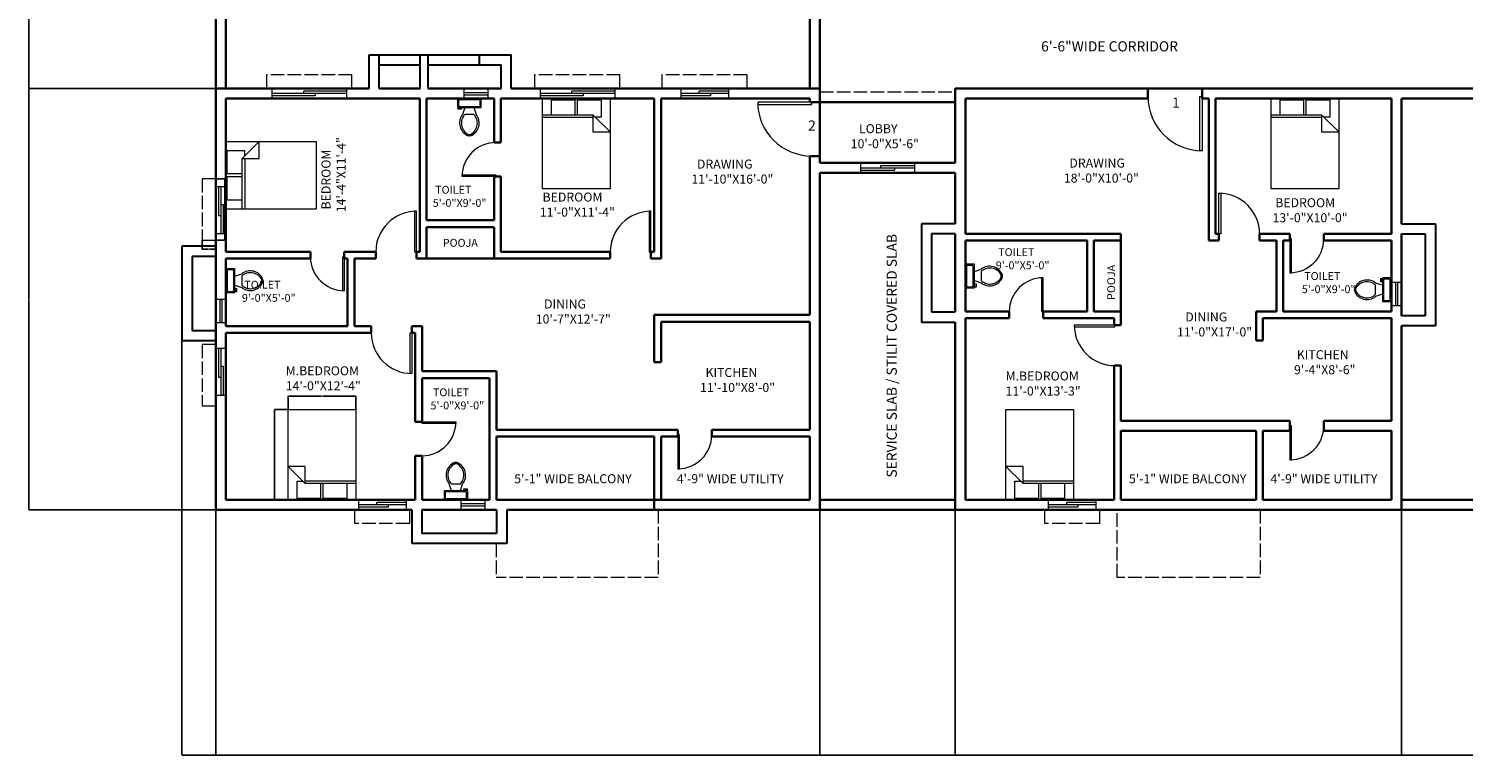
# Model space of a CAD drawing. Units: inches. Extents: x -69 to 2453, y 4803 to 7122.
# Tile 1 of 9: x -69 to 1203, y 4803 to 5448. Entities that reach past the tile are written whole.
import ezdxf

# ---------------------------------------------------------------- set-up
doc = ezdxf.new("R2010")
doc.units = ezdxf.units.IN
doc.linetypes.add('ACAD_ISO02W100', pattern=[15, 12, -3])
for name, color, linetype, lineweight in [('A-ANNO-DIMS', 2, 'Continuous', 18), ('A-ANNO-IDEN', 2, 'Continuous', 18), ('A-AREA-IDEN', 7, 'Continuous', 18), ('A-DOOR', 3, 'Continuous', 18), ('A-FLOR-FIXT', 9, 'Continuous', 18), ('A-FLOR-OVHD', 8, 'ACAD_ISO02W100', 13), ('A-FURN', 8, 'Continuous', 18), ('A-GLAZ', 244, 'Continuous', 18), ('A-WALL', 7, 'Continuous', 35), ('A-WALL-SRVC', 7, 'Continuous', 30)]:
    doc.layers.add(name, color=color, linetype=linetype, lineweight=lineweight)
doc.styles.get("Standard").update_dxf_attribs({"font": 'arial.ttf'})
doc.dimstyles.get("Standard").update_dxf_attribs({"dimtxt": 0.18, "dimasz": 0.18, "dimexe": 0.18, "dimexo": 0.0625, "dimgap": 0.09, "dimtad": 0, "dimtih": 1, "dimtoh": 1, "dimdec": 4, "dimzin": 0, "dimdsep": 46, "dimtxsty": 'Standard', "dimcen": 0.09, "dimadec": 0, "dimazin": 0, "dimtfac": 1, "dimtdec": 4, "dimtofl": 0, "dimtmove": 0, "dimatfit": 3, "dimfxl": 1, "dimtolj": 1, "dimtzin": 0, "dimarcsym": 0})

# ---------------------------------------------------------------- blocks, each defined once
blk = doc.blocks.new('*U2')
for p, q in [((-40, 0), (-40, 6)), ((0, 0), (0, 6))]:
    blk.add_line(p, q)
blk.add_lwpolyline([(0, 0), (0, -40), (-1.75, -40), (-1.75, 0)], close=True)
blk.add_arc((0, 0), 40, 180, 270)
blk = doc.blocks.new('*U4')
for p, q in [((0, 0), (0, -6)), ((-40, 0), (-40, -6))]:
    blk.add_line(p, q)
blk.add_lwpolyline([(0, 0), (0, 40), (-1.75, 40), (-1.75, 0)], close=True)
blk.add_arc((0, 0), 40, 90, 180)
blk = doc.blocks.new('*U3')
for p, q in [((0, 0), (0, 6)), ((40, 0), (40, 6))]:
    blk.add_line(p, q)
blk.add_lwpolyline([(0, 0), (0, -40), (1.75, -40), (1.75, 0)], close=True)
blk.add_arc((0, 0), 40, 270, 360)
blk = doc.blocks.new('*U6')
for p, q in [((-40, 0), (-40, 6)), ((0, 0), (0, 6))]:
    blk.add_line(p, q)
blk.add_lwpolyline([(0, 0), (0, -40), (-1.75, -40), (-1.75, 0)], close=True)
blk.add_arc((0, 0), 40, 180, 270)
blk = doc.blocks.new('*U17')
for p, q in [((0, 0), (0, 6)), ((40, 0), (40, 6))]:
    blk.add_line(p, q)
blk.add_lwpolyline([(0, 0), (0, -40), (1.75, -40), (1.75, 0)], close=True)
blk.add_arc((0, 0), 40, 270, 0)
blk = doc.blocks.new('*U5')
for p, q in [((0, 0), (0, -6)), ((40, 0), (40, -6))]:
    blk.add_line(p, q)
blk.add_lwpolyline([(0, 0), (0, 40), (1.75, 40), (1.75, 0)], close=True)
blk.add_arc((0, 0), 40, 0, 90)
blk = doc.blocks.new('*U21')
for p, q in [((-40, 0), (-40, -6)), ((0, 0), (0, -6))]:
    blk.add_line(p, q)
blk.add_lwpolyline([(0, 0), (0, 40), (-1.75, 40), (-1.75, 0)], close=True)
blk.add_arc((0, 0), 40, 90, 180)
blk = doc.blocks.new('Bed - Queen')
for p, q in [((0, -80.00003), (0, 0)), ((0, 0), (59.99999, 0)), ((59.99999, 0), (59.99999, -80.00003)), ((7.99999, -1.2), (28.79998, -1.2)), ((7.99999, -14.4), (7.99999, -1.2)), ((28.79998, -1.2), (28.79998, -14.4)), ((31.19999, -1.2), (51.99999, -1.2)), ((31.19999, -14.4), (31.19999, -1.2)), ((51.99999, -1.2), (51.99999, -16.4)), ((0, -14.4), (44.8, -14.4)), ((44.8, -16.8), (0, -16.8)), ((59.99999, -29.6), (44.8, -14.4)), ((44.8, -14.4), (44.8, -29.6)), ((51.99999, -16.4), (46.79936, -16.4)), ((44.8, -29.6), (59.99999, -29.6)), ((59.99999, -80.00003), (0, -80.00003))]:
    blk.add_line(p, q)
blk = doc.blocks.new('*U33')
for p, q in [((-10, -8.5), (-8, -8.5)), ((-10, -9.5), (-10, -8.5)), ((-7, -9.5), (-10, -9.5)), ((-8, -8.5), (-8, -8)), ((-7, -8), (-7, -9.5)), ((-4, -8), (-6, -14)), ((4, -8), (6, -14)), ((9.5, -6), (9.5, -2)), ((4, -14), (-4, -14))]:
    blk.add_line(p, q)
blk.add_lwpolyline([(10.5, -8), (10.5, 0), (-10.5, 0), (-10.5, -8)], close=True)
for points in [[(-9.5, -2), (-9.5, -6)], [(8.5, -1), (-8.5, -1)], [(-8.5, -7), (8.5, -7)]]:
    blk.add_lwpolyline(points)
for centre, radius, start, end in [((-8.6, -1.9), 0.884, 81.8699, 188.1301), ((-8.6, -6.1), 0.884, 171.8699, 278.1301), ((8.6, -1.9), 0.884, 351.8699, 98.1301), ((8.6, -6.1), 0.884, 261.8699, 8.1301), ((3.5, -21.6), 12.2, 141.4691, 247.9714), ((4.2, -21.8), 11.3, 136.3677, 238.9468), ((-3.5, -21.6), 12.2, 292.0284, 38.5307), ((-4.2, -21.8), 11.3, 301.053, 43.6321), ((0, -27.9), 4, 245.7318, 294.2682), ((0, -29), 4, 254.8605, 285.1395)]:
    blk.add_arc(centre, radius, start, end)
blk = doc.blocks.new('WINDOW-VENT-21IN')
for p, q in [((0, 5.5), (21, 5.5)), ((0, 3.5), (21, 3.5))]:
    blk.add_line(p, q)
blk.add_lwpolyline([(0, 9), (21, 9), (21, 0), (0, 0)], close=True)
blk = doc.blocks.new('WINDOW-SLIDING-42IN')
for p, q in [((2.5, 42), (2.5, 16)), ((4.5, 42), (4.5, 0)), ((4.5, 26), (6.5, 26)), ((6.5, 26), (6.5, 0)), ((4.5, 16), (2.5, 16))]:
    blk.add_line(p, q)
blk.add_lwpolyline([(0, 42), (9, 42), (9, 0), (0, 0)], close=True)
blk = doc.blocks.new('WINDOW-SLIDING-66IN')
for p, q in [((66, 4.5), (0, 4.5)), ((38, 2.5), (0, 2.5)), ((66, 6.5), (28, 6.5)), ((28, 4.5), (28, 6.5)), ((38, 4.5), (38, 2.5))]:
    blk.add_line(p, q)
blk.add_lwpolyline([(66, 9), (66, 0), (0, 0), (0, 9)], close=True)
blk = doc.blocks.new('SUNSHADE-54IN')
for p, q in [((12, 54.3), (0, 54.3)), ((0, 54.3), (0, 0)), ((0, 0), (12, 0))]:
    blk.add_line(p, q)
blk = doc.blocks.new('SUNSHADE-48IN')
for p, q in [((0, 0), (0, 12)), ((48.4, 0), (0, 0)), ((48.4, 12), (48.4, 0))]:
    blk.add_line(p, q)
blk = doc.blocks.new('SUNSHADE-76IN')
for p, q in [((75.7, 12), (0, 12)), ((0, 12), (0, 0)), ((75.7, 0), (75.7, 12))]:
    blk.add_line(p, q)
blk = doc.blocks.new('SERVICE-BAY-87IN')
for p, q in [((30, 87.2), (0, 87.2)), ((0, 87.2), (0, 0)), ((30, 78.2), (9, 78.2)), ((9, 78.2), (9, 9)), ((0, 0), (30, 0)), ((9, 9), (30, 9))]:
    blk.add_line(p, q)
blk = doc.blocks.new('*D51')
at = {"layer": 'A-ANNO-DIMS', "color": 0, "lineweight": -2, "transparency": 16777216}
for p, q in [((160.6, 5109.7), (148.5, 5109.7)), ((148.7, 5109.5), (148.7, 5069.9)), ((148.7, 5029.9), (148.7, 5069.5)), ((160.6, 5029.7), (148.5, 5029.7))]:
    blk.add_line(p, q, dxfattribs=at)
at = {"layer": 'A-ANNO-DIMS', "color": 0, "transparency": 16777216}
for points in [[(148.7, 5109.5), (148.7, 5109.5), (148.7, 5109.7)], [(148.7, 5029.9), (148.7, 5029.9), (148.7, 5029.7)]]:
    blk.add_solid(points, dxfattribs=at)
at = {"layer": 'Defpoints', "color": 0, "transparency": 16777216}
for p in [(160.7, 5109.7), (148.7, 5029.7), (160.7, 5029.7)]:
    blk.add_point(p, dxfattribs=at)
at = {"layer": 'A-ANNO-DIMS', "color": 0, "transparency": 16777216, "insert": (148.7, 5069.7), "char_height": 0.18, "attachment_point": 5}
blk.add_mtext('\\A1;QUEEN BED 80 TYP.', dxfattribs=at)
blk = doc.blocks.new('*D52')
at = {"layer": 'A-ANNO-DIMS', "color": 0, "lineweight": -2, "transparency": 16777216}
for p, q in [((160.7, 5109.8), (160.7, 5121.9)), ((160.9, 5121.7), (190.2, 5121.7)), ((220.5, 5121.7), (191.2, 5121.7)), ((220.7, 5109.8), (220.7, 5121.9))]:
    blk.add_line(p, q, dxfattribs=at)
at = {"layer": 'A-ANNO-DIMS', "color": 0, "transparency": 16777216}
for points in [[(160.9, 5121.7), (160.9, 5121.7), (160.7, 5121.7)], [(220.5, 5121.7), (220.5, 5121.7), (220.7, 5121.7)]]:
    blk.add_solid(points, dxfattribs=at)
at = {"layer": 'Defpoints', "color": 0, "transparency": 16777216}
for p in [(160.7, 5121.7), (160.7, 5109.7), (220.7, 5109.7)]:
    blk.add_point(p, dxfattribs=at)
at = {"layer": 'A-ANNO-DIMS', "color": 0, "transparency": 16777216, "insert": (190.7, 5121.7), "char_height": 0.18, "attachment_point": 5}
blk.add_mtext('\\A1;60 TYP.', dxfattribs=at)
blk = doc.blocks.new('*D59')
at = {"layer": 'A-ANNO-DIMS', "color": 0, "lineweight": -2, "transparency": 16777216}
for p, q in [((96.6, 5314.5), (104.8, 5314.5)), ((104.7, 5314.3), (104.7, 5287.5)), ((104.7, 5260.4), (104.7, 5287.2)), ((96.6, 5260.2), (104.8, 5260.2))]:
    blk.add_line(p, q, dxfattribs=at)
at = {"layer": 'A-ANNO-DIMS', "color": 0, "transparency": 16777216}
for points in [[(104.6, 5314.3), (104.7, 5314.3), (104.7, 5314.5)], [(104.6, 5260.4), (104.7, 5260.4), (104.7, 5260.2)]]:
    blk.add_solid(points, dxfattribs=at)
at = {"layer": 'Defpoints', "color": 0, "transparency": 16777216}
for p in [(96.5, 5314.5), (104.7, 5314.5), (96.5, 5260.2)]:
    blk.add_point(p, dxfattribs=at)
at = {"layer": 'A-ANNO-DIMS', "color": 0, "transparency": 16777216, "insert": (104.7, 5287.4), "char_height": 0.18, "attachment_point": 5}
blk.add_mtext('\\A1;SUNSHADE 54 TYP.', dxfattribs=at)
blk = doc.blocks.new('*D60')
at = {"layer": 'A-ANNO-DIMS', "color": 0, "lineweight": -2, "transparency": 16777216}
for p, q in [((84.5, 5260.1), (84.5, 5251.9)), ((96.5, 5260.1), (96.5, 5251.9)), ((84.7, 5252), (90, 5252)), ((96.3, 5252), (91, 5252))]:
    blk.add_line(p, q, dxfattribs=at)
at = {"layer": 'A-ANNO-DIMS', "color": 0, "transparency": 16777216}
for points in [[(84.7, 5252.1), (84.7, 5252), (84.5, 5252)], [(96.3, 5252.1), (96.3, 5252), (96.5, 5252)]]:
    blk.add_solid(points, dxfattribs=at)
at = {"layer": 'Defpoints', "color": 0, "transparency": 16777216}
for p in [(84.5, 5260.2), (96.5, 5260.2), (96.5, 5252)]:
    blk.add_point(p, dxfattribs=at)
at = {"layer": 'A-ANNO-DIMS', "color": 0, "transparency": 16777216, "insert": (90.5, 5252), "char_height": 0.18, "attachment_point": 5}
blk.add_mtext('\\A1;12 TYP.', dxfattribs=at)
blk = doc.blocks.new('*D81')
at = {"layer": 'A-ANNO-DIMS', "color": 0, "lineweight": -2, "transparency": 16777216}
for p, q in [((96.5, 5020.7), (96.5, 4802.8)), ((632.5, 5020.7), (632.5, 4802.8)), ((96.7, 4803), (364.2, 4803)), ((632.3, 4803), (364.8, 4803))]:
    blk.add_line(p, q, dxfattribs=at)
at = {"layer": 'A-ANNO-DIMS', "color": 0, "transparency": 16777216}
for points in [[(96.7, 4803), (96.7, 4802.9), (96.5, 4803)], [(632.3, 4803), (632.3, 4802.9), (632.5, 4803)]]:
    blk.add_solid(points, dxfattribs=at)
at = {"layer": 'Defpoints', "color": 0, "transparency": 16777216}
for p in [(96.5, 5020.7), (632.5, 5020.7), (632.5, 4803)]:
    blk.add_point(p, dxfattribs=at)
at = {"layer": 'A-ANNO-DIMS', "color": 0, "transparency": 16777216, "insert": (364.5, 4803), "char_height": 0.18, "attachment_point": 5}
blk.add_mtext('\\A1;536', dxfattribs=at)
blk = doc.blocks.new('*D82')
at = {"layer": 'A-ANNO-DIMS', "color": 0, "lineweight": -2, "transparency": 16777216}
for p, q in [((632.5, 5020.7), (632.5, 4802.8)), ((752.5, 5020.7), (752.5, 4802.8)), ((632.7, 4803), (692.2, 4803)), ((752.3, 4803), (692.8, 4803))]:
    blk.add_line(p, q, dxfattribs=at)
at = {"layer": 'A-ANNO-DIMS', "color": 0, "transparency": 16777216}
for points in [[(632.7, 4803), (632.7, 4802.9), (632.5, 4803)], [(752.3, 4803), (752.3, 4802.9), (752.5, 4803)]]:
    blk.add_solid(points, dxfattribs=at)
at = {"layer": 'Defpoints', "color": 0, "transparency": 16777216}
for p in [(632.5, 5020.7), (752.5, 5020.7), (752.5, 4803)]:
    blk.add_point(p, dxfattribs=at)
at = {"layer": 'A-ANNO-DIMS', "color": 0, "transparency": 16777216, "insert": (692.5, 4803), "char_height": 0.18, "attachment_point": 5}
blk.add_mtext('\\A1;120', dxfattribs=at)
blk = doc.blocks.new('*D83')
at = {"layer": 'A-ANNO-DIMS', "color": 0, "lineweight": -2, "transparency": 16777216}
for p, q in [((752.5, 5020.7), (752.5, 4802.8)), ((1148.5, 5020.7), (1148.5, 4802.8)), ((752.7, 4803), (950.2, 4803)), ((1148.3, 4803), (950.8, 4803))]:
    blk.add_line(p, q, dxfattribs=at)
at = {"layer": 'A-ANNO-DIMS', "color": 0, "transparency": 16777216}
for points in [[(752.7, 4803), (752.7, 4802.9), (752.5, 4803)], [(1148.3, 4803), (1148.3, 4802.9), (1148.5, 4803)]]:
    blk.add_solid(points, dxfattribs=at)
at = {"layer": 'Defpoints', "color": 0, "transparency": 16777216}
for p in [(752.5, 5020.7), (1148.5, 5020.7), (1148.5, 4803)]:
    blk.add_point(p, dxfattribs=at)
at = {"layer": 'A-ANNO-DIMS', "color": 0, "transparency": 16777216, "insert": (950.5, 4803), "char_height": 0.18, "attachment_point": 5}
blk.add_mtext('\\A1;396', dxfattribs=at)
blk = doc.blocks.new('*D84')
at = {"layer": 'A-ANNO-DIMS', "color": 0, "lineweight": -2, "transparency": 16777216}
for p, q in [((1148.5, 5020.7), (1148.5, 4802.8)), ((1277.5, 5020.7), (1277.5, 4802.8)), ((1148.7, 4803), (1212.7, 4803)), ((1277.3, 4803), (1213.3, 4803))]:
    blk.add_line(p, q, dxfattribs=at)
at = {"layer": 'A-ANNO-DIMS', "color": 0, "transparency": 16777216}
for points in [[(1148.7, 4803), (1148.7, 4802.9), (1148.5, 4803)], [(1277.3, 4803), (1277.3, 4802.9), (1277.5, 4803)]]:
    blk.add_solid(points, dxfattribs=at)
at = {"layer": 'Defpoints', "color": 0, "transparency": 16777216}
for p in [(1148.5, 5020.7), (1277.5, 5020.7), (1277.5, 4803)]:
    blk.add_point(p, dxfattribs=at)
at = {"layer": 'A-ANNO-DIMS', "color": 0, "transparency": 16777216, "insert": (1213, 4803), "char_height": 0.18, "attachment_point": 5}
blk.add_mtext('\\A1;129', dxfattribs=at)
blk = doc.blocks.new('*D95')
at = {"layer": 'A-ANNO-DIMS', "color": 0, "lineweight": -2, "transparency": 16777216}
for p, q in [((96.509262, 5020.652777), (96.509262, 4802.785277)), ((2286.509262, 4977.652777), (2286.509262, 4802.785277)), ((96.689262, 4802.965277), (1191.149262, 4802.965277)), ((2286.329262, 4802.965277), (1191.869262, 4802.965277))]:
    blk.add_line(p, q, dxfattribs=at)
at = {"layer": 'A-ANNO-DIMS', "color": 0, "transparency": 16777216}
for points in [[(96.689262, 4802.995277), (96.689262, 4802.935277), (96.509262, 4802.965277)], [(2286.329262, 4802.995277), (2286.329262, 4802.935277), (2286.509262, 4802.965277)]]:
    blk.add_solid(points, dxfattribs=at)
at = {"layer": 'Defpoints', "color": 0, "transparency": 16777216}
for p in [(96.509262, 5020.715277), (2286.509262, 4977.715277), (2286.509262, 4802.965277)]:
    blk.add_point(p, dxfattribs=at)
at = {"layer": 'A-ANNO-DIMS', "color": 0, "transparency": 16777216, "insert": (1191.509262, 4802.965277), "char_height": 0.18, "attachment_point": 5}
blk.add_mtext('\\A1;2190', dxfattribs=at)
blk = doc.blocks.new('*D97')
at = {"layer": 'A-ANNO-DIMS', "color": 0, "lineweight": -2, "transparency": 16777216}
for p, q in [((96.4, 5394.7), (-69.4, 5394.7)), ((-69.2, 5394.5), (-69.2, 5207.9)), ((-69.2, 5020.9), (-69.2, 5207.5)), ((96.4, 5020.7), (-69.4, 5020.7))]:
    blk.add_line(p, q, dxfattribs=at)
at = {"layer": 'A-ANNO-DIMS', "color": 0, "transparency": 16777216}
for points in [[(-69.3, 5394.5), (-69.2, 5394.5), (-69.2, 5394.7)], [(-69.3, 5020.9), (-69.2, 5020.9), (-69.2, 5020.7)]]:
    blk.add_solid(points, dxfattribs=at)
at = {"layer": 'Defpoints', "color": 0, "transparency": 16777216}
for p in [(-69.2, 5394.7), (96.5, 5394.7), (96.5, 5020.7)]:
    blk.add_point(p, dxfattribs=at)
at = {"layer": 'A-ANNO-DIMS', "color": 0, "transparency": 16777216, "insert": (-69.2, 5207.7), "char_height": 0.18, "attachment_point": 5}
blk.add_mtext('\\A1;374', dxfattribs=at)
blk = doc.blocks.new('*D98')
at = {"layer": 'A-ANNO-DIMS', "color": 0, "lineweight": -2, "transparency": 16777216}
for p, q in [((96.4, 5514.7), (-69.4, 5514.7)), ((-69.2, 5514.5), (-69.2, 5454.9)), ((-69.2, 5394.9), (-69.2, 5454.5)), ((96.4, 5394.7), (-69.4, 5394.7))]:
    blk.add_line(p, q, dxfattribs=at)
at = {"layer": 'A-ANNO-DIMS', "color": 0, "transparency": 16777216}
for points in [[(-69.3, 5514.5), (-69.2, 5514.5), (-69.2, 5514.7)], [(-69.3, 5394.9), (-69.2, 5394.9), (-69.2, 5394.7)]]:
    blk.add_solid(points, dxfattribs=at)
at = {"layer": 'Defpoints', "color": 0, "transparency": 16777216}
for p in [(-69.2, 5514.7), (96.5, 5514.7), (96.5, 5394.7)]:
    blk.add_point(p, dxfattribs=at)
at = {"layer": 'A-ANNO-DIMS', "color": 0, "transparency": 16777216, "insert": (-69.2, 5454.7), "char_height": 0.18, "attachment_point": 5}
blk.add_mtext('\\A1;120', dxfattribs=at)
blk = doc.blocks.new('*D105')
at = {"layer": 'A-ANNO-DIMS', "color": 0, "lineweight": -2, "transparency": 16777216}
for p, q in [((66.509262, 5170.610035), (66.509262, 4802.785277)), ((2316.509262, 5140.587945), (2316.509262, 4802.785277)), ((66.689262, 4802.965277), (1191.149262, 4802.965277)), ((2316.329262, 4802.965277), (1191.869262, 4802.965277))]:
    blk.add_line(p, q, dxfattribs=at)
at = {"layer": 'A-ANNO-DIMS', "color": 0, "transparency": 16777216}
for points in [[(66.689262, 4802.995277), (66.689262, 4802.935277), (66.509262, 4802.965277)], [(2316.329262, 4802.995277), (2316.329262, 4802.935277), (2316.509262, 4802.965277)]]:
    blk.add_solid(points, dxfattribs=at)
at = {"layer": 'Defpoints', "color": 0, "transparency": 16777216}
for p in [(66.509262, 5170.672535), (2316.509262, 5140.650445), (2316.509262, 4802.965277)]:
    blk.add_point(p, dxfattribs=at)
at = {"layer": 'A-ANNO-DIMS', "color": 0, "transparency": 16777216, "insert": (1191.509262, 4802.965277), "char_height": 0.18, "attachment_point": 5}
blk.add_mtext('\\A1;2250', dxfattribs=at)

msp = doc.modelspace()

# ---------------------------------------------------------------- linework, layer by layer
at = {"layer": 'A-FLOR-OVHD'}
for p, q in [((632.5, 5391.7), (752.5, 5391.7)), ((489, 5020.7), (489, 4960.7)), ((896.1, 4960.7), (896.1, 5020.7)), ((1023, 5020.7), (1023, 4960.7)), ((345.4, 4990.7), (345.4, 4960.7)), ((489, 4960.7), (345.4, 4960.7)), ((1023, 4960.7), (896.1, 4960.7))]:
    msp.add_line(p, q, dxfattribs=at)
at = {"layer": 'A-GLAZ'}
for p, q in [((668.5, 5328.7), (668.5, 5319.7)), ((668.5, 5324.2), (716.5, 5324.2)), ((668.5, 5322.2), (698.5, 5322.2)), ((686.5, 5326.2), (716.5, 5326.2)), ((686.5, 5324.2), (686.5, 5326.2)), ((698.5, 5324.2), (698.5, 5322.2)), ((716.5, 5328.7), (716.5, 5319.7))]:
    msp.add_line(p, q, dxfattribs=at)
at = {"layer": 'A-WALL'}
for p, q in [((632.5, 6021.7), (632.5, 5328.7)), ((96.5, 5659.3), (96.5, 5020.7)), ((105.5, 5514.7), (105.5, 5394.7)), ((623.5, 5514.7), (623.5, 5394.7)), ((96.5, 5394.7), (232.6, 5394.7)), ((105.5, 5385.7), (277.5, 5385.7)), ((105.5, 5385.7), (105.5, 5249.7)), ((241.6, 5394.7), (277.8, 5394.7)), ((277.5, 5385.7), (277.5, 5249.7)), ((283.5, 5385.7), (283.5, 5277.7)), ((283.5, 5385.7), (343.5, 5385.7)), ((284.9, 5394.7), (349.7, 5394.7)), ((343.5, 5385.7), (343.5, 5346.7)), ((349.5, 5385.7), (349.5, 5346.7)), ((349.5, 5385.7), (485.5, 5385.7)), ((358.7, 5394.7), (632.5, 5394.7)), ((485.5, 5385.7), (485.5, 5249.7)), ((491.5, 5385.7), (623.5, 5385.7)), ((491.5, 5385.7), (491.5, 5243.7)), ((623.5, 5385.7), (623.5, 5382.7)), ((752.5, 5394.7), (752.5, 5328.7)), ((752.5, 5394.7), (1673.5, 5394.7)), ((761.5, 5385.7), (761.5, 5265.7)), ((761.5, 5385.7), (923.5, 5385.7)), ((923.5, 5385.7), (923.5, 5394.7)), ((971.5, 5385.7), (971.5, 5394.7)), ((971.5, 5385.7), (977.5, 5385.7)), ((977.5, 5385.7), (977.5, 5259.7)), ((983.5, 5385.7), (983.5, 5265.7)), ((983.5, 5385.7), (1139.5, 5385.7)), ((1139.5, 5385.7), (1139.5, 5265.7)), ((1148.5, 5385.7), (1277.5, 5385.7)), ((1148.5, 5385.7), (1148.5, 5274.7)), ((623.5, 5382.7), (752.5, 5382.7)), ((343.5, 5346.7), (349.5, 5346.7)), ((623.5, 5334.7), (632.5, 5334.7)), ((623.5, 5334.7), (623.5, 5193.7)), ((632.5, 5328.7), (752.5, 5328.7)), ((343.5, 5316.7), (349.5, 5316.7)), ((343.5, 5316.7), (343.5, 5277.7)), ((349.5, 5316.7), (349.5, 5249.7)), ((632.5, 5319.7), (752.5, 5319.7)), ((632.5, 5319.7), (632.5, 5020.7)), ((752.5, 5319.7), (752.5, 5274.6)), ((283.5, 5277.7), (343.5, 5277.7)), ((283.5, 5271.7), (343.5, 5271.7)), ((283.5, 5271.7), (283.5, 5243.7)), ((343.5, 5271.7), (343.5, 5243.7)), ((752.5, 5265.6), (752.5, 5196.4)), ((761.5, 5265.7), (899.5, 5265.7)), ((761.5, 5259.7), (869.5, 5259.7)), ((761.5, 5259.7), (761.5, 5196.7)), ((869.5, 5259.7), (869.5, 5196.7)), ((875.5, 5259.7), (875.5, 5196.7)), ((875.5, 5259.7), (899.5, 5259.7)), ((899.5, 5265.7), (899.5, 5184.7)), ((977.5, 5259.7), (986.5, 5259.7)), ((983.5, 5265.7), (986.5, 5265.7)), ((986.5, 5265.7), (986.5, 5259.7)), ((1022.5, 5265.7), (1022.5, 5259.7)), ((1022.5, 5265.7), (1049.5, 5265.7)), ((1022.5, 5259.7), (1037.5, 5259.7)), ((1037.5, 5259.7), (1037.5, 5196.7)), ((1043.5, 5259.7), (1043.5, 5196.7)), ((1043.5, 5259.7), (1049.5, 5259.7)), ((1049.5, 5259.7), (1049.5, 5265.7)), ((1079.5, 5259.7), (1079.5, 5265.7)), ((1079.5, 5265.7), (1139.5, 5265.7)), ((1079.5, 5259.7), (1139.5, 5259.7)), ((1139.5, 5259.7), (1139.5, 5196.7)), ((1148.5, 5265.7), (1148.5, 5193)), ((105.5, 5249.7), (180.5, 5249.7)), ((105.5, 5243.7), (180.5, 5243.7)), ((105.5, 5243.7), (105.5, 5183.7)), ((180.5, 5243.7), (180.5, 5249.7)), ((210.5, 5243.7), (210.5, 5249.7)), ((210.5, 5249.7), (238.5, 5249.7)), ((210.5, 5243.7), (213.5, 5243.7)), ((213.5, 5243.7), (213.5, 5183.7)), ((219.5, 5243.7), (219.5, 5183.7)), ((219.5, 5243.7), (238.5, 5243.7)), ((238.5, 5249.7), (238.5, 5243.7)), ((274.5, 5249.7), (274.5, 5243.7)), ((274.5, 5249.7), (277.5, 5249.7)), ((274.5, 5243.7), (446.5, 5243.7)), ((349.5, 5249.7), (446.5, 5249.7)), ((446.5, 5249.7), (446.5, 5243.7)), ((482.5, 5249.7), (482.5, 5243.7)), ((482.5, 5249.7), (485.5, 5249.7)), ((482.5, 5243.7), (491.5, 5243.7)), ((485.5, 5193.7), (623.5, 5193.7)), ((485.5, 5193.7), (485.5, 5151.7)), ((761.5, 5196.7), (800.5, 5196.7)), ((800.5, 5196.7), (800.5, 5190.7)), ((830.5, 5196.7), (830.5, 5190.7)), ((830.5, 5196.7), (869.5, 5196.7)), ((875.5, 5196.7), (899.5, 5196.7)), ((1019.5, 5196.7), (1037.5, 5196.7)), ((1019.5, 5196.7), (1019.5, 5170.9)), ((1043.5, 5196.7), (1139.5, 5196.7)), ((105.5, 5183.7), (213.5, 5183.7)), ((219.5, 5183.7), (234.5, 5183.7)), ((234.5, 5177.7), (234.5, 5183.7)), ((270.5, 5177.7), (270.5, 5183.7)), ((270.5, 5183.7), (279.5, 5183.7)), ((279.5, 5183.7), (279.5, 5143.7)), ((491.5, 5187.7), (623.5, 5187.7)), ((491.5, 5187.7), (491.5, 5151.7)), ((623.5, 5187.7), (623.5, 5091.7)), ((752.5, 5187.4), (752.5, 5020.7)), ((761.5, 5190.7), (800.5, 5190.7)), ((761.5, 5190.7), (761.5, 5029.7)), ((830.5, 5190.7), (893.5, 5190.7)), ((893.5, 5190.7), (893.5, 5184.7)), ((893.5, 5184.7), (899.5, 5184.7)), ((1025.5, 5190.7), (1139.5, 5190.7)), ((1025.5, 5190.7), (1025.5, 5170.9)), ((1139.5, 5190.7), (1139.5, 5099.7)), ((1148.5, 5184), (1148.5, 5020.7)), ((105.5, 5177.7), (234.5, 5177.7)), ((105.5, 5177.7), (105.5, 5029.7)), ((270.5, 5177.7), (273.5, 5177.7)), ((273.5, 5177.7), (273.5, 5098.7)), ((1025.5, 5170.9), (1019.5, 5170.9)), ((279.5, 5143.7), (345.5, 5143.7)), ((345.5, 5143.7), (345.5, 5091.7)), ((491.5, 5151.7), (485.5, 5151.7)), ((893.5, 5148.7), (899.5, 5148.7)), ((893.5, 5148.7), (893.5, 5029.7)), ((899.5, 5148.7), (899.5, 5099.7)), ((279.5, 5137.7), (339.5, 5137.7)), ((279.5, 5137.7), (279.5, 5098.7)), ((339.5, 5137.7), (339.5, 5029.7)), ((279.5, 5098.7), (273.5, 5098.7)), ((345.5, 5091.7), (506.5, 5091.7)), ((506.5, 5085.7), (506.5, 5091.7)), ((536.5, 5085.7), (536.5, 5091.7)), ((536.5, 5091.7), (623.5, 5091.7)), ((899.5, 5099.7), (1049.5, 5099.7)), ((1049.5, 5090.7), (1049.5, 5099.7)), ((1079.5, 5090.7), (1079.5, 5099.7)), ((1079.5, 5099.7), (1139.5, 5099.7)), ((345.5, 5085.7), (485.5, 5085.7)), ((345.5, 5085.7), (345.5, 5029.7)), ((485.5, 5085.7), (485.5, 5020.7)), ((491.5, 5085.7), (491.5, 5029.7)), ((491.5, 5085.7), (506.5, 5085.7)), ((536.5, 5085.7), (623.5, 5085.7)), ((623.5, 5085.7), (623.5, 5029.7)), ((899.5, 5090.7), (1019.5, 5090.7)), ((899.5, 5090.7), (899.5, 5029.7)), ((1019.5, 5090.7), (1019.5, 5029.7)), ((1025.5, 5090.7), (1049.5, 5090.7)), ((1025.5, 5090.7), (1025.5, 5029.7)), ((1079.5, 5090.7), (1139.5, 5090.7)), ((1139.5, 5090.7), (1139.5, 5029.7)), ((279.5, 5068.7), (273.5, 5068.7)), ((273.5, 5068.7), (273.5, 5029.7)), ((279.5, 5068.7), (279.5, 5029.7)), ((105.5, 5029.7), (273.5, 5029.7)), ((279.5, 5029.7), (339.5, 5029.7)), ((345.5, 5029.7), (623.5, 5029.7)), ((632.5, 5029.7), (752.5, 5029.7)), ((761.5, 5029.7), (893.5, 5029.7)), ((899.5, 5029.7), (1019.5, 5029.7)), ((1025.5, 5029.7), (1139.5, 5029.7)), ((1148.5, 5029.7), (1277.5, 5029.7)), ((96.5, 5020.7), (270.4, 5020.7)), ((279.4, 5020.7), (345.7, 5020.7)), ((354.7, 5020.7), (1793.5, 5020.7))]:
    msp.add_line(p, q, dxfattribs=at)
at = {"layer": 'A-WALL-SRVC'}
for p, q in [((232.6, 5424.7), (358.7, 5424.7)), ((232.6, 5394.7), (232.6, 5424.7)), ((241.6, 5394.7), (241.6, 5424.7)), ((277.8, 5394.7), (277.8, 5424.7)), ((284.9, 5394.7), (284.9, 5424.7)), ((330.6, 5415.7), (330.6, 5424.7)), ((358.7, 5394.7), (358.7, 5424.7)), ((241.6, 5415.7), (277.8, 5415.7)), ((284.9, 5415.7), (349.7, 5415.7)), ((349.7, 5394.7), (349.7, 5415.7)), ((1148.5, 5274.7), (1178.5, 5274.7)), ((1178.5, 5274.7), (1178.5, 5184)), ((1148.5, 5265.7), (1169.5, 5265.7)), ((1169.5, 5265.7), (1169.5, 5193)), ((66.5, 5254.6), (66.5, 5170.7)), ((96.5, 5254.6), (66.5, 5254.6)), ((96.5, 5245.6), (75.5, 5245.6)), ((75.5, 5245.6), (75.5, 5179.7)), ((1169.5, 5193), (1148.5, 5193)), ((1178.5, 5184), (1148.5, 5184)), ((96.5, 5170.7), (66.5, 5170.7)), ((96.5, 5179.7), (75.5, 5179.7)), ((270.4, 5020.7), (270.4, 4990.7)), ((279.4, 5020.7), (279.4, 4999.7)), ((345.7, 5020.7), (345.7, 4999.7)), ((354.7, 5020.7), (354.7, 4990.7)), ((354.7, 4990.7), (270.4, 4990.7)), ((345.7, 4999.7), (279.4, 4999.7))]:
    msp.add_line(p, q, dxfattribs=at)

# ---------------------------------------------------------------- block references
at = {"layer": 'A-DOOR'}
for name, p, xscale, yscale, zscale in [('*U6', (971.5, 5387.5), 1.199999999999977, 1.199999999999977, 1.199999999999977), ('*U5', (986.5, 5265.7), 0.9, 0.9, 0.9), ('*U4', (274.5, 5249.7), 0.9, 0.9, 0.9), ('*U4', (482.5, 5249.7), 0.9, 0.9, 0.9), ('*U3', (1049.5, 5261.2), 0.7500000000000029, 0.7500000000000029, 0.7500000000000029), ('*U2', (210.5, 5245.2), 0.75, 0.75, 0.75), ('*U21', (830.5, 5196.7), 0.7500000000000029, 0.7500000000000029, 0.7500000000000029), ('*U2', (270.5, 5177.7), 0.9, 0.9, 0.9), ('*U3', (506.5, 5087.2), 0.7500000000000029, 0.7500000000000029, 0.7500000000000029), ('*U3', (1049.5, 5095.2), 0.7500000000000029, 0.7500000000000029, 0.7500000000000029)]:
    msp.add_blockref(name, p, dxfattribs=dict(at, xscale=xscale, yscale=yscale, zscale=zscale))
for name, p, xscale, yscale, zscale, rotation in [('*U3', (625.3, 5382.7), 1.199999999999977, 1.199999999999977, 1.199999999999977, 270.0000000000001), ('*U2', (345, 5316.7), 0.75, 0.75, 0.75, 270.0000000000001), ('*U17', (894.1, 5184.7), 0.9, 0.9, 0.9, 270), ('*U5', (279.5, 5098.7), 0.75, 0.75, 0.75, 270.0000000000001)]:
    msp.add_blockref(name, p, dxfattribs=dict(at, xscale=xscale, yscale=yscale, zscale=zscale, rotation=rotation))
at = {"layer": 'A-FLOR-FIXT'}
msp.add_blockref('*U33', (321.5, 5385.7), dxfattribs=at)
for p, rotation in [((105.5, 5224.1), 89.99999999999999), ((761.5, 5228.2), 89.99999999999999), ((1139.5, 5216), 270), ((309.5, 5029.7), 180)]:
    msp.add_blockref('*U33', p, dxfattribs=dict(at, rotation=rotation))
at = {"layer": 'A-FLOR-OVHD'}
for name, p in [('SUNSHADE-76IN', (141.6, 5394.7)), ('SUNSHADE-76IN', (379.4, 5394.7)), ('SUNSHADE-76IN', (492.2, 5394.7)), ('SUNSHADE-54IN', (84.5, 5260.2)), ('SUNSHADE-54IN', (84.5, 5113.1)), ('SUNSHADE-48IN', (220, 5008.7)), ('SUNSHADE-48IN', (832, 5008.7))]:
    msp.add_blockref(name, p, dxfattribs=at)
at = {"layer": 'A-FURN'}
for p in [(386.3, 5385.7), (1032.7, 5385.7)]:
    msp.add_blockref('Bed - Queen', p, dxfattribs=at)
for p, rotation in [((105.5, 5287.7), 89.99999999999999), ((220.7, 5029.7), 180), ((857.5, 5029.7), 180)]:
    msp.add_blockref('Bed - Queen', p, dxfattribs=dict(at, rotation=rotation))
at = {"layer": 'A-GLAZ'}
for name, p in [('WINDOW-SLIDING-66IN', (146.6, 5385.7)), ('WINDOW-VENT-21IN', (316.8, 5385.7)), ('WINDOW-SLIDING-66IN', (384.5, 5385.7)), ('WINDOW-SLIDING-42IN', (96.5, 5265.8)), ('WINDOW-SLIDING-42IN', (96.5, 5122.3)), ('WINDOW-VENT-21IN', (314.1, 5020.7))]:
    msp.add_blockref(name, p, dxfattribs=at)
for name, p, rotation in [('WINDOW-SLIDING-42IN', (509.3, 5394.7), 269.9999999999985), ('WINDOW-VENT-21IN', (1139.5, 5222.7), 269.999999999998), ('WINDOW-VENT-21IN', (96.5, 5207.7), 270.0000000000005), ('WINDOW-SLIDING-42IN', (223.5, 5029.7), 269.9999999999984), ('WINDOW-SLIDING-42IN', (835.4, 5029.7), 270.0000000000007)]:
    msp.add_blockref(name, p, dxfattribs=dict(at, rotation=rotation))
at = {"layer": 'A-WALL-SRVC'}
msp.add_blockref('SERVICE-BAY-87IN', (722.5, 5187.4), dxfattribs=at)

# ---------------------------------------------------------------- texts
at = {"layer": 'A-ANNO-IDEN', "char_height": 8, "attachment_point": 1}
for s, width, insert in [('{\\H1.125x;1} ', 9.054, (944.9, 5386.6)), ('{\\H1.125x;2} ', 10.499, (622, 5366.3))]:
    msp.add_mtext_dynamic_manual_height_columns(s, width=width, gutter_width=12.5, heights=[0], dxfattribs=dict(at, insert=insert))
at = {"layer": 'A-AREA-IDEN', "attachment_point": 1}
for s, width, heights, insert, char_height in [('6\'-6"WIDE CORRIDOR', 131.057, [0], (828.7, 5436.6), 9), ('   LOBBY\\P10\'-0"X5\'-6"', 57.156, [0], (659.8, 5363), 8), ('  DRAWING\\P18\'-0"X10\'-0"', 66.094, [21.6], (848.9, 5332.5), 8), ('  DRAWING\\P11\'-10"X16\'-0"', 64.991, [0], (518.5, 5331.6), 8), (' TOILET\\P5\'-0"X9\'-0"', 51.03, [0], (289, 5308.3), 7), (' BEDROOM\\P11\'-0"X11\'-4"', 64.991, [0], (384, 5302.3), 8), (' BEDROOM\\P13\'-0"X10\'-0"', 64.991, [0], (1034, 5297.3), 8), ('POOJA', 33.919, [0], (297.9, 5261.2), 7), (' TOILET\\P9\'-0"X5\'-0"', 45.2, [0], (788.5, 5252.9), 7), (' TOILET\\P5\'-0"X9\'-0"', 45.2, [0], (1060, 5231.7), 7), (' TOILET\\P9\'-0"X5\'-0"', 45.2, [0], (119.7, 5224), 7), ('   DINING\\P10\'-7"X12\'-7"', 63.236, [0], (380.4, 5207.4), 8), ('   DINING\\P11\'-0"X17\'-0"', 63.236, [0], (949.3, 5195.9), 8), (' KITCHEN\\P9\'-4"X8\'-6"', 58.128, [0], (1053.1, 5162.4), 8), ('M.BEDROOM\\P14\'-0"X12\'-4"', 69.603, [0], (158.6, 5148.1), 8), ('  KITCHEN\\P11\'-10"X8\'-0"', 63.236, [0], (526.1, 5146.6), 8), ('M.BEDROOM\\P11\'-0"X13\'-3"', 69.603, [0], (797.2, 5143.5), 8), (' TOILET\\P5\'-0"X9\'-0"', 45.251, [0], (287, 5128.5), 7), ('5\'-1" WIDE BALCONY', 114.375, [0], (361.3, 5052.3), 8), ('4\'-9" WIDE UTILITY', 99.552, [0], (505.5, 5052.3), 8), ('5\'-1" WIDE BALCONY', 114.375, [0], (906.6, 5052.3), 8), ('4\'-9" WIDE UTILITY', 99.552, [0], (1032.2, 5052.3), 8)]:
    msp.add_mtext_dynamic_manual_height_columns(s, width=width, gutter_width=12.5, heights=heights, dxfattribs=dict(at, insert=insert, char_height=char_height))
at = {"layer": 'A-AREA-IDEN', "attachment_point": 1, "rotation": 90}
for s, width, insert, char_height in [(' BEDROOM\\P14\'-4"X11\'-4"', 64.991, (190.3, 5284.9), 8), ('SERVICE SLAB / STILIT COVERED SLAB', 250.4, (691.7, 5049.3), 9), ('POOJA', 33.919, (887.4, 5207), 7)]:
    msp.add_mtext_dynamic_manual_height_columns(s, width=width, gutter_width=12.5, heights=[0], dxfattribs=dict(at, insert=insert, char_height=char_height))

# ---------------------------------------------------------------- dimensions: what is measured, and where the dimension line sits
at = {"layer": 'A-ANNO-DIMS'}
for base, p1, p2, picture, middle in [((-69.2, 5514.7), (96.5, 5394.7), (96.5, 5514.7), '*D98', (-69.2, 5454.7)), ((-69.2, 5394.7), (96.5, 5020.7), (96.5, 5394.7), '*D97', (-69.2, 5207.7))]:
    dim = msp.add_linear_dim(base=base, p1=p1, p2=p2, angle=90, dimstyle='Standard', override={"dimdec": 0, "dimlfac": 1, "dimrnd": 0, "dimzin": 0, "dimdsep": 46, "dimlunit": 2}, dxfattribs=at)
    dim.commit()
    dim.dimension.update_dxf_attribs({"geometry": picture, "text_midpoint": middle})
for base, p1, p2, angle, text, picture, middle in [((104.7, 5314.5), (96.5, 5260.2), (96.5, 5314.5), 90, 'SUNSHADE <> TYP.', '*D59', (104.7, 5287.4)), ((160.7, 5121.7), (220.7, 5109.7), (160.7, 5109.7), 180, '<> TYP.', '*D52', (190.7, 5121.7)), ((148.7, 5029.7), (160.7, 5109.7), (160.7, 5029.7), 270, 'QUEEN BED <> TYP.', '*D51', (148.7, 5069.7))]:
    dim = msp.add_linear_dim(base=base, p1=p1, p2=p2, angle=angle, text=text, dimstyle='Standard', override={"dimdec": 0, "dimlfac": 1, "dimrnd": 0, "dimzin": 0, "dimdsep": 46, "dimlunit": 2}, dxfattribs=at)
    dim.commit()
    dim.dimension.update_dxf_attribs({"geometry": picture, "text_midpoint": middle})
dim = msp.add_linear_dim(base=(96.5, 5252), p1=(84.5, 5260.2), p2=(96.5, 5260.2), text='<> TYP.', dimstyle='Standard', override={"dimdec": 0, "dimlfac": 1, "dimrnd": 0, "dimzin": 0, "dimdsep": 46, "dimlunit": 2}, dxfattribs=at)
dim.commit()
dim.dimension.update_dxf_attribs({"geometry": '*D60', "text_midpoint": (90.5, 5252)})
for base, p1, p2, picture, middle in [((2316.5, 4803), (66.5, 5170.7), (2316.5, 5140.7), '*D105', (1191.5, 4803)), ((632.5, 4803), (96.5, 5020.7), (632.5, 5020.7), '*D81', (364.5, 4803)), ((2286.5, 4803), (96.5, 5020.7), (2286.5, 4977.7), '*D95', (1191.5, 4803)), ((752.5, 4803), (632.5, 5020.7), (752.5, 5020.7), '*D82', (692.5, 4803)), ((1148.5, 4803), (752.5, 5020.7), (1148.5, 5020.7), '*D83', (950.5, 4803)), ((1277.5, 4803), (1148.5, 5020.7), (1277.5, 5020.7), '*D84', (1213, 4803))]:
    dim = msp.add_linear_dim(base=base, p1=p1, p2=p2, dimstyle='Standard', override={"dimdec": 0, "dimlfac": 1, "dimrnd": 0, "dimzin": 0, "dimdsep": 46, "dimlunit": 2}, dxfattribs=at)
    dim.commit()
    dim.dimension.update_dxf_attribs({"geometry": picture, "text_midpoint": middle})

doc.saveas('drawing.dxf')
